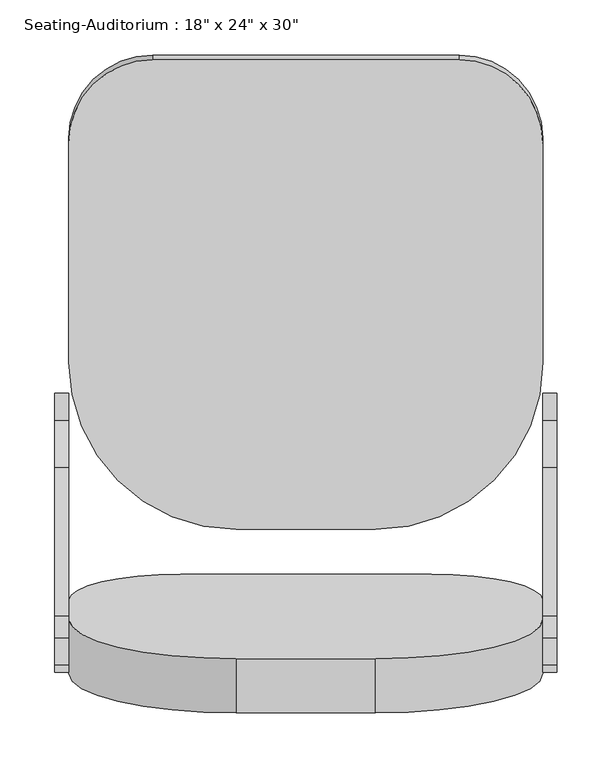
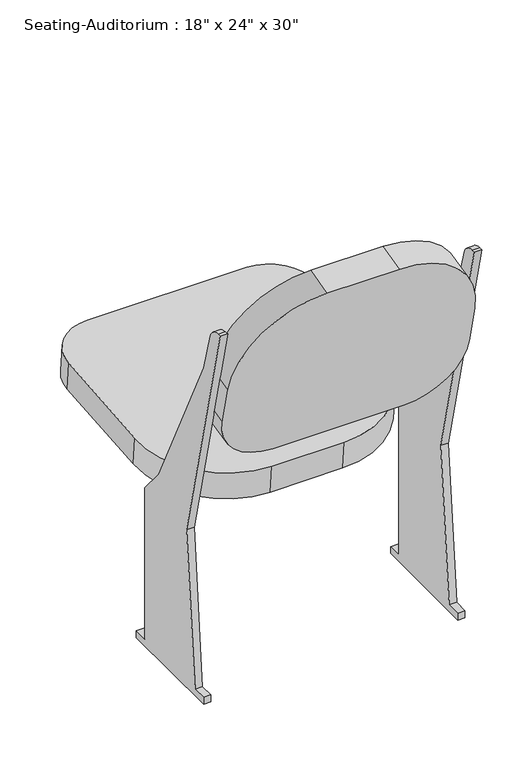
"""IFC4 building model written with IfcOpenShell, lengths in millimetres: furniture geometry."""

from ifc_helpers import new_model, si_unit, point, frame, frame_2d, origin, place, context, project, spatial, polyline, circle_curve, trimmed, segment, composite_curve, outline, extrude, source, transform, mapped, element, save


def furniture_eb3a3c23(model_context):
    return source(origin(), model_context, "Body", "SweptSolid", [
        extrude(outline(composite_curve([segment(polyline([(-13.3245902, 12.7), (12.0754098, 12.7), (37.4754098, 292.1), (-64.1245902, 711.2), (-57.883846, 711.2)]), True, "CONTINUOUS"), segment(trimmed(circle_curve(frame_2d((-57.883846, 685.8)), 25.4), [point((-57.883846, 711.2))], [point((-33.4611378, 692.7779166))], False, "CARTESIAN"), True, "CONTINUOUS"), segment(polyline([(-33.4611378, 692.7779166), (-13.3245902, 622.3), (121.8491486, 342.9), (164.4754098, 292.1), (164.4754098, 12.7), (189.8754098, 12.7), (189.8754098, 0.0), (-13.3245902, 0.0), (-13.3245902, 12.7)]), True, "CONTINUOUS")], self_intersect=False)), frame((376.6278689, 0.0, 0.0), z_axis=(1.0, 0.0, 0.0), x_axis=(0.0, 1.0, 0.0)), (0.0, 0.0, 1.0), 12.7),
        extrude(outline(composite_curve([segment(polyline([(-13.3245902, 0.0), (-13.3245902, 12.7), (12.0754098, 12.7), (37.4754098, 292.1), (-64.1245902, 711.2), (-57.883846, 711.2)]), True, "CONTINUOUS"), segment(trimmed(circle_curve(frame_2d((-57.883846, 685.8)), 25.4), [point((-57.883846, 711.2))], [point((-33.4611378, 692.7779166))], False, "CARTESIAN"), True, "CONTINUOUS"), segment(polyline([(-33.4611378, 692.7779166), (-13.3245902, 622.3), (121.8491486, 342.9), (164.4754098, 292.1), (164.4754098, 12.7), (189.8754098, 12.7), (189.8754098, 0.0), (-13.3245902, 0.0)]), True, "CONTINUOUS")], self_intersect=False)), frame((-67.8721311, 0.0, 0.0), z_axis=(1.0, 0.0, 0.0), x_axis=(0.0, 1.0, 0.0)), (0.0, 0.0, 1.0), 12.7),
        extrude(outline(composite_curve([segment(trimmed(circle_curve(frame_2d((0.0, -76.2)), 76.2), [point((0.0, 0.0))], [point((76.2, -76.2))], False, "CARTESIAN"), True, "CONTINUOUS"), segment(polyline([(76.2, -76.2), (76.2, -276.4123505)]), True, "CONTINUOUS"), segment(trimmed(circle_curve(frame_2d((-76.2, -276.4123505)), 152.4), [point((76.2, -276.4123505))], [point((-76.2, -428.8123506))], False, "CARTESIAN"), True, "CONTINUOUS"), segment(polyline([(-76.2, -428.8123506), (-203.2, -428.8123506)]), True, "CONTINUOUS"), segment(trimmed(circle_curve(frame_2d((-203.2, -276.4123505)), 152.4), [point((-203.2, -428.8123506))], [point((-355.6, -276.4123505))], False, "CARTESIAN"), True, "CONTINUOUS"), segment(polyline([(-355.6, -276.4123505), (-355.6, -76.2)]), True, "CONTINUOUS"), segment(trimmed(circle_curve(frame_2d((-279.4, -76.2)), 76.2), [point((-355.6, -76.2))], [point((-279.4, 0.0))], False, "CARTESIAN"), True, "CONTINUOUS"), segment(polyline([(-279.4, 0.0), (0.0, 0.0)]), True, "CONTINUOUS")], self_intersect=False)), frame((300.4278689, 497.5245173, 321.2380213), z_axis=(0.0, -0.08715574274765496, 0.9961946980917459), x_axis=(1.0, 0.0, 0.0)), (0.0, 0.0, 1.0), 50.8),
        extrude(outline(composite_curve([segment(polyline([(0.0, 0.0), (127.0, 0.0)]), True, "CONTINUOUS"), segment(trimmed(circle_curve(frame_2d((127.0, -152.4)), 152.4), [point((127.0, 0.0))], [point((279.4, -152.4))], False, "CARTESIAN"), True, "CONTINUOUS"), segment(polyline([(279.4, -152.4), (279.4, -224.0588601)]), True, "CONTINUOUS"), segment(trimmed(circle_curve(frame_2d((177.8, -224.0588601)), 101.6), [point((279.4, -224.0588601))], [point((177.8, -325.6588601))], False, "CARTESIAN"), True, "CONTINUOUS"), segment(polyline([(177.8, -325.6588601), (-50.8, -325.6588601)]), True, "CONTINUOUS"), segment(trimmed(circle_curve(frame_2d((-50.8, -224.0588601)), 101.6), [point((-50.8, -325.6588601))], [point((-152.4, -224.0588601))], False, "CARTESIAN"), True, "CONTINUOUS"), segment(polyline([(-152.4, -224.0588601), (-152.4, -152.4)]), True, "CONTINUOUS"), segment(trimmed(circle_curve(frame_2d((0.0, -152.4)), 152.4), [point((-152.4, -152.4))], [point((0.0, 0.0))], False, "CARTESIAN"), True, "CONTINUOUS")], self_intersect=False)), frame((224.2278689, -101.3396919, 755.9484479), z_axis=(0.0, 0.9717404775047361, 0.23605178325712217), x_axis=(-1.0, 0.0, 0.0)), (0.0, 0.0, 1.0), 50.8),
    ])


if __name__ == "__main__":
    model = new_model("IFC4")
    model_context = context("Model", 3, world=origin())
    ifc_project = project(units=[si_unit("LENGTHUNIT", "METRE", prefix="MILLI")], contexts=[model_context])
    site = spatial("IfcSite", under=ifc_project)
    building = spatial("IfcBuilding", under=site)
    placement = place(None, origin())
    furniture_shape = furniture_eb3a3c23(model_context)
    element("IfcFurniture", 1, ObjectType="Seating-Auditorium : 18\" x 24\" x 30\"", at=placement, inside=building, context=model_context, shape_type="MappedRepresentation", body=[
        mapped(furniture_shape, transform((0.0, 0.0, 0.0), x_axis=(1.0, 0.0, 0.0), y_axis=(0.0, 1.0, 0.0), z_axis=(0.0, 0.0, 1.0))),
    ])
    save(model, "model.ifc")

# Revit data of these elements
# Type "Seating-Auditorium : 18\" x 24\" x 30\""
#   Assembly Code = "E2020200"
#   Seat Material = Linen, Beige
#   Frame Material = Steel, Paint Finish, Dark Gray, Matte
#   Default Elevation = 0
# Element 1 (IfcFurniture, "Seating-Auditorium : 18\" x 24\" x 30\"")
#   Materials on its faces: "Steel, Paint Finish, Dark Gray, Matte", "Linen, Beige"
# Materials
#   "Linen, Beige": class "Textile", colour RGB 249 239 230, transparency 0, Description = "Linen, beige", Cost = 0
#   "Steel, Paint Finish, Dark Gray, Matte": class "Metal", colour RGB 0 0 0, transparency 0, Description = "Steel, paint finish, dark gray, matte", Cost = 0
